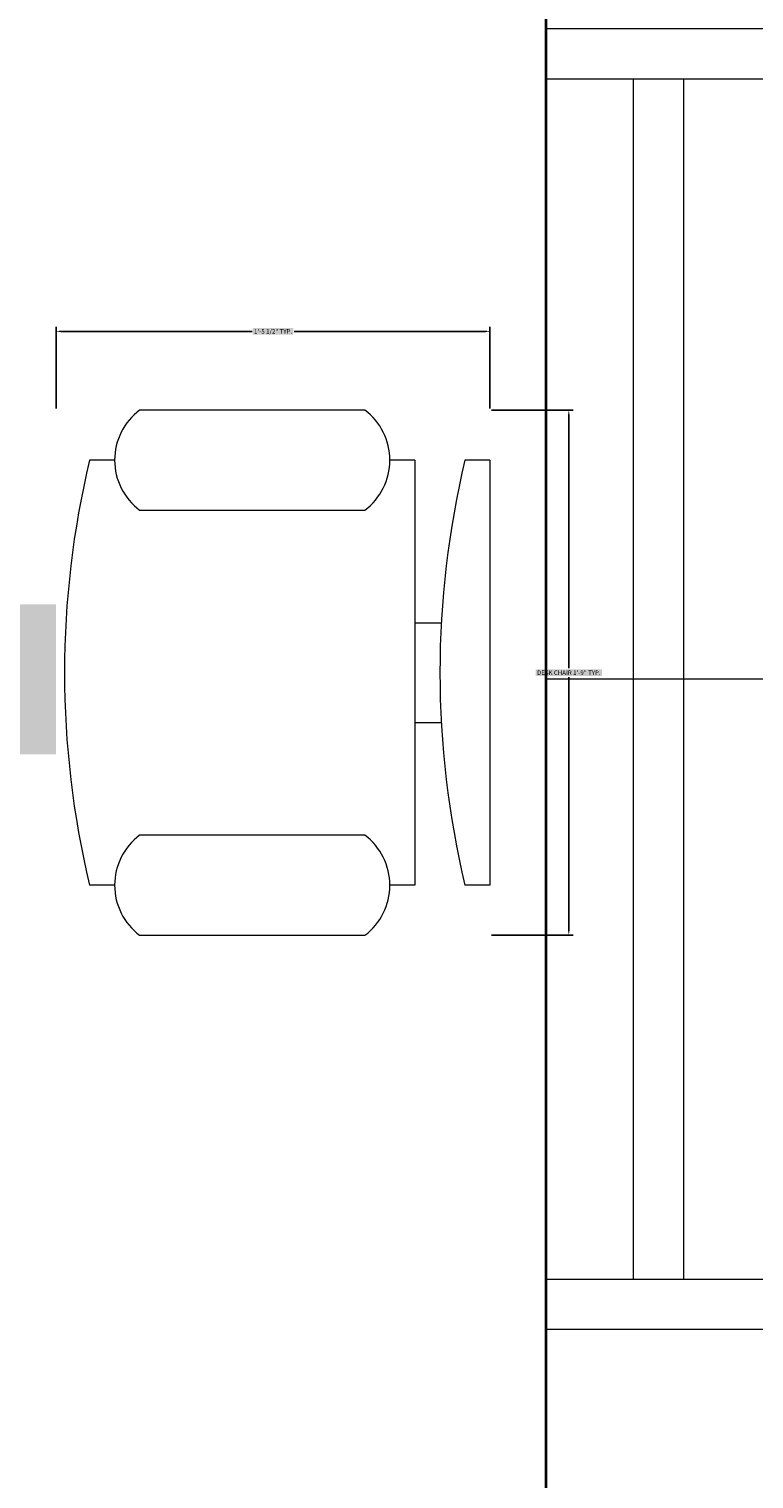
# Model space of a CAD drawing. Units: inches. Extents: x -128 to 854, y -395 to 398.
# Tile 46 of 61: x 284 to 313, y 236 to 294. Entities that reach past the tile are written whole.
import ezdxf

# ---------------------------------------------------------------- set-up
doc = ezdxf.new("R2010")
doc.units = ezdxf.units.IN
doc.header["$MEASUREMENT"] = 0
for name, color, linetype, lineweight in [('A-ANNO-DIMS', 2, 'Continuous', 18), ('A-FURN', 8, 'Continuous', 18), ('A-GLAZ', 220, 'Continuous', 18), ('A-WALL', 4, 'Continuous', 35)]:
    doc.layers.add(name, color=color, linetype=linetype, lineweight=lineweight)
doc.styles.get("Standard").update_dxf_attribs({"font": 'arial.ttf'})
doc.dimstyles.get("Standard").update_dxf_attribs({"dimtxt": 0.18, "dimasz": 0.18, "dimexe": 0.18, "dimexo": 0.0625, "dimgap": 0.09, "dimtad": 0, "dimtih": 1, "dimtoh": 1, "dimdec": 1, "dimzin": 0, "dimdsep": 46, "dimlunit": 4, "dimtxsty": 'Standard', "dimcen": 0.09, "dimclrd": 1, "dimclre": 2, "dimclrt": 6, "dimadec": 0, "dimazin": 0, "dimtfac": 1, "dimtdec": 1, "dimtofl": 0, "dimtmove": 0, "dimatfit": 3, "dimfxl": 1, "dimtfill": 2, "dimtfillclr": 3, "dimtolj": 1, "dimtzin": 0, "dimarcsym": 0})

# ---------------------------------------------------------------- blocks, each defined once
blk = doc.blocks.new('Chair - Desk')
for p, q in [((-8.5, 0), (-8.5, -1)), ((-8.5, 0), (8.5, 0)), ((8.5, 0), (8.5, -1)), ((-2, -3), (-2, -1.9355)), ((2, -1.9576), (2, -3)), ((-8.5, -3), (-8.5, -4)), ((-8.5, -3), (8.5, -3)), ((8.5, -3), (8.5, -4)), ((-10.5, -5), (-10.5, -14)), ((-6.5, -14), (-6.5, -5)), ((6.5, -5), (6.5, -14)), ((10.5, -14), (10.5, -5)), ((-8.5, -15), (-8.5, -16)), ((8.5, -15), (8.5, -16))]:
    blk.add_line(p, q)
for centre, radius, start, end in [((0, 34.625), 36.625, 256.5803, 283.4197), ((-8.5, -6.5), 2.5, 36.8699, 143.1301), ((8.5, -6.5), 2.5, 36.8699, 143.1301), ((-8.5, -12.5), 2.5, 216.8699, 323.1301), ((8.5, -12.5), 2.5, 216.8699, 323.1301), ((0, 19.625), 36.625, 256.5803, 283.4197)]:
    blk.add_arc(centre, radius, start, end)
blk = doc.blocks.new('*D53')
at = {"layer": 'A-ANNO-DIMS', "color": 0, "lineweight": -2, "transparency": 16777216}
for p, q in [((304.81, 339.741), (280.297, 339.741)), ((280.477, 334.741), (280.477, 269.839)), ((280.477, 200.741), (280.477, 265.642)), ((304.81, 195.741), (280.297, 195.741))]:
    blk.add_line(p, q, dxfattribs=at)
at = {"layer": 'A-ANNO-DIMS', "color": 0, "transparency": 16777216}
for points in [[(279.644, 334.741), (281.311, 334.741), (280.477, 339.741)], [(279.644, 200.741), (281.311, 200.741), (280.477, 195.741)]]:
    blk.add_solid(points, dxfattribs=at)
at = {"layer": 'Defpoints', "color": 0, "transparency": 16777216}
for p in [(280.477, 339.741), (304.873, 339.741), (304.873, 195.741)]:
    blk.add_point(p, dxfattribs=at)
at = {"layer": 'A-ANNO-DIMS', "color": 0, "transparency": 16777216, "insert": (280.477, 267.741), "char_height": 4, "attachment_point": 5, "bg_fill": 1, "box_fill_scale": 1.25, "bg_fill_color": 3, "bg_fill_transparency": 0}
blk.add_mtext("\\A1;12'", dxfattribs=at)
blk = doc.blocks.new('WIN-48IN')
for p, q in [((9, 52), (0, 52)), ((9, 50), (0, 50)), ((3.5, 50), (3.5, 2)), ((5.5, 50), (5.5, 2)), ((9, 26), (0, 26)), ((9, 2), (0, 2)), ((9, 0), (0, 0))]:
    blk.add_line(p, q)
blk = doc.blocks.new('*D85')
at = {"layer": 'A-ANNO-DIMS', "color": 2, "lineweight": -2, "transparency": 16777216}
for p, q in [((302.707, 278.501), (305.975, 278.501)), ((302.707, 257.501), (305.975, 257.501))]:
    blk.add_line(p, q, dxfattribs=at)
at = {"layer": 'A-ANNO-DIMS', "color": 1, "lineweight": -2, "transparency": 16777216}
for p, q in [((305.795, 278.321), (305.795, 268.184)), ((305.795, 257.681), (305.795, 267.818))]:
    blk.add_line(p, q, dxfattribs=at)
at = {"layer": 'A-ANNO-DIMS', "color": 1, "transparency": 16777216}
for points in [[(305.765, 278.321), (305.825, 278.321), (305.795, 278.501)], [(305.765, 257.681), (305.825, 257.681), (305.795, 257.501)]]:
    blk.add_solid(points, dxfattribs=at)
at = {"layer": 'Defpoints', "color": 0, "transparency": 16777216}
for p in [(302.645, 278.501), (302.645, 257.501), (305.795, 257.501)]:
    blk.add_point(p, dxfattribs=at)
at = {"layer": 'A-ANNO-DIMS', "color": 6, "transparency": 16777216, "insert": (305.795, 268.001), "char_height": 0.18, "attachment_point": 5, "bg_fill": 1, "box_fill_scale": 1.25, "bg_fill_color": 3, "bg_fill_transparency": 0}
blk.add_mtext('\\A1;DESK CHAIR 1\'-9" TYP.', dxfattribs=at)
blk = doc.blocks.new('*D86')
at = {"layer": 'A-ANNO-DIMS', "color": 2, "lineweight": -2, "transparency": 16777216}
for p, q in [((285.311, 278.563), (285.311, 281.831)), ((302.645, 278.563), (302.645, 281.831))]:
    blk.add_line(p, q, dxfattribs=at)
at = {"layer": 'A-ANNO-DIMS', "color": 1, "lineweight": -2, "transparency": 16777216}
for p, q in [((285.491, 281.651), (293.138, 281.651)), ((302.465, 281.651), (294.818, 281.651))]:
    blk.add_line(p, q, dxfattribs=at)
at = {"layer": 'A-ANNO-DIMS', "color": 1, "transparency": 16777216}
for points in [[(285.491, 281.681), (285.491, 281.621), (285.311, 281.651)], [(302.465, 281.681), (302.465, 281.621), (302.645, 281.651)]]:
    blk.add_solid(points, dxfattribs=at)
at = {"layer": 'Defpoints', "color": 0, "transparency": 16777216}
for p in [(302.645, 281.651), (285.311, 278.501), (302.645, 278.501)]:
    blk.add_point(p, dxfattribs=at)
at = {"layer": 'A-ANNO-DIMS', "color": 6, "transparency": 16777216, "insert": (293.978, 281.651), "char_height": 0.18, "attachment_point": 5, "bg_fill": 1, "box_fill_scale": 1.25, "bg_fill_color": 3, "bg_fill_transparency": 0}
blk.add_mtext('\\A1;1\'-5 1/2" TYP.', dxfattribs=at)

msp = doc.modelspace()

# ---------------------------------------------------------------- linework, layer by layer
at = {"layer": 'A-WALL'}
msp.add_line((304.873, 339.741), (304.873, 195.741), dxfattribs=at)

# ---------------------------------------------------------------- block references
at = {"layer": 'A-FURN', "rotation": 270}
msp.add_blockref('Chair - Desk', (302.645, 268.001), dxfattribs=at)
at = {"layer": 'A-GLAZ'}
msp.add_blockref('WIN-48IN', (304.873, 241.741), dxfattribs=at)

# ---------------------------------------------------------------- dimensions: what is measured, and where the dimension line sits
at = {"layer": 'A-ANNO-DIMS'}
dim = msp.add_linear_dim(base=(280.477, 339.741), p1=(304.873, 195.741), p2=(304.873, 339.741), angle=90, dimstyle='Standard', override={"dimtxt": 4, "dimasz": 5, "dimclrd": 0, "dimclre": 0, "dimclrt": 0}, dxfattribs=at)
dim.commit()
dim.dimension.update_dxf_attribs({"geometry": '*D53', "text_midpoint": (280.477, 267.741)})
dim = msp.add_linear_dim(base=(302.645, 281.651), p1=(285.311, 278.501), p2=(302.645, 278.501), text='<> TYP.', dimstyle='Standard', override={"dimdec": 1, "dimlfac": 1, "dimrnd": 0, "dimzin": 1, "dimdsep": 46, "dimlunit": 4, "dimfrac": 2}, dxfattribs=at)
dim.commit()
dim.dimension.update_dxf_attribs({"geometry": '*D86', "text_midpoint": (293.978, 281.651)})
dim = msp.add_linear_dim(base=(305.795, 257.501), p1=(302.645, 278.501), p2=(302.645, 257.501), angle=270, text='DESK CHAIR <> TYP.', dimstyle='Standard', override={"dimdec": 1, "dimlfac": 1, "dimrnd": 0, "dimzin": 1, "dimdsep": 46, "dimlunit": 4, "dimfrac": 2}, dxfattribs=at)
dim.commit()
dim.dimension.update_dxf_attribs({"geometry": '*D85', "text_midpoint": (305.795, 268.001)})

doc.saveas('drawing.dxf')
